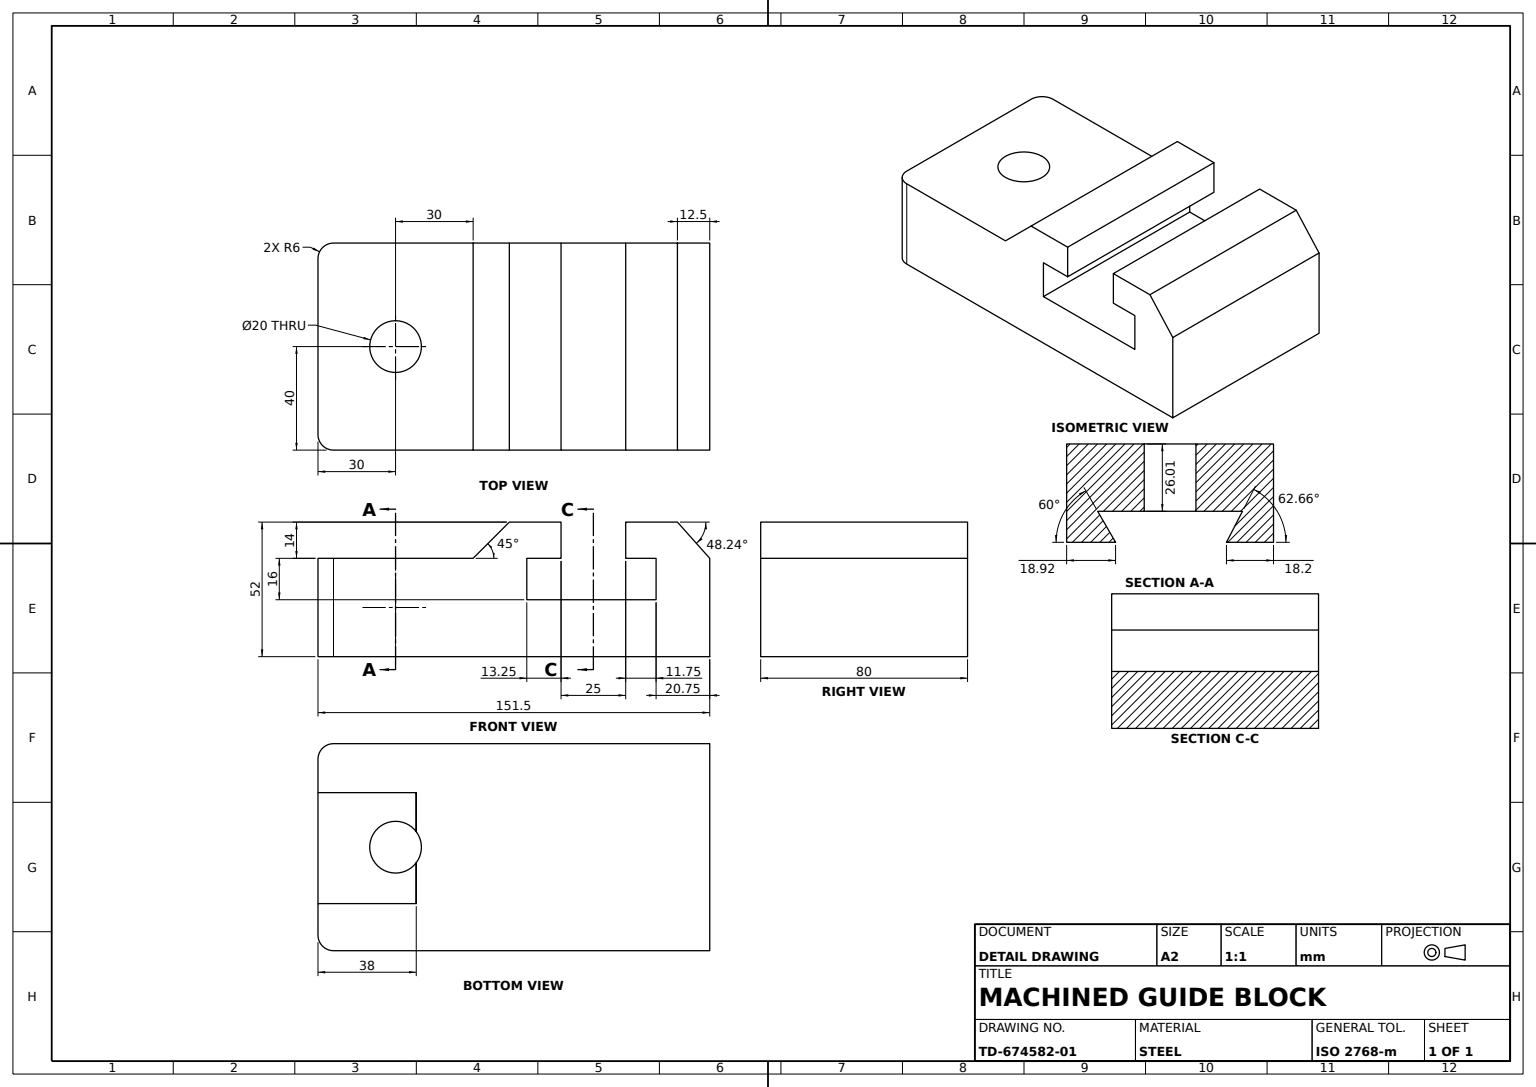
SolidWorks part; units mm, degrees
material "Plain Carbon Steel"
ref_plane "Front Plane" through (0, 0, 0) normal (0, 0, 1) x (1, 0, 0)
ref_plane "Top Plane" through (0, 0, 0) normal (0, 1, 0) x (1, 0, 0)
ref_plane "Right Plane" through (0, 0, 0) normal (1, 0, 0) x (0, 0, -1)
sketch "Base Profile Sketch" plane through (0, 0, 0) normal (0, 0, 1) x (1, 0, 0)
  line L0 (54, 0) -> (144, 0)
  line L1 (131.5, 52) -> (144, 38)
  line L2 (52.5, 0) -> (-1.5, 0)
  line L3 (52.5, 0) -> (54, 0)
  line L4 (144, 38) -> (144, 22)
  line L5 (54, 0) -> (144, 0)
  line L6 (86.5, 52) -> (86.5, 38)
  line L7 (111.5, 52) -> (111.5, 38)
  line L8 (52.5, 0) -> (144, 0)
  line L9 (86.5, 52) -> (66.5, 52)
  line L10 (111.5, 52) -> (131.5, 52)
  line L11 (144, 22) -> (144, 0)
  line L12 (52.5, 38) -> (66.5, 52)
  line L13 (0, 0) -> (0, 0.1905)
  line L14 (52.5, 0) -> (54, 0)
  line L15 (-1.5, 38) -> (-1.5, 0)
  line L16 (86.5, 38) -> (73.25, 38)
  line L17 (73.25, 38) -> (86.5, 38)
  line L18 (123.25, 38) -> (123.25, 22)
  line L19 (123.25, 22) -> (73.25, 22)
  line L20 (73.25, 22) -> (73.25, 38)
  line L21 (111.5, 38) -> (123.25, 38)
  line L22 (52.5, 38) -> (-1.5, 38)
  arc A0 (-1.5, 0) -> (0, 0.1905) centre (-1.5, 6) ccw
  dimension "D1" = 6
  dimension "D2" = 1.5
  dimension "D3" = 54
  dimension "D4" = 55.5
  dimension "D5" = 68
  dimension "D6" = 74.75
  dimension "D7" = 88
  dimension "D8" = 113
  dimension "D9" = 124.75
  dimension "D10" = 145.5
  dimension "D11" = 22
  dimension "D12" = 38
  dimension "D13" = 52
extrude "Base Body" add sketch "Base Profile Sketch" along normal blind 80 contours L15 A0 L13 L2 L3 L0 L11 L4 L1 L10 L7 L21 L18 L19 L20 L16 L6 L9 L12 L22
sketch "Raised Block Sketch" plane through (0, 38, 0) normal (0, 1, 0) x (1, 0, 0)
  line L0 (-1.5, 0) -> (-1.5, -6)
  line L1 (-1.5, -80) -> (-1.5, 0) construction
  line L2 (-1.5, -80) -> (-1.5, -74)
  line L3 (-1.5, -6) -> (-1.5, -74)
  line L4 (-7.5, -6) -> (-7.5, -74)
  arc A0 (-1.5, 0) -> (-7.5, -6) centre (-1.5, -6) ccw
  arc A1 (-7.5, -74) -> (-1.5, -80) centre (-1.5, -74) ccw
  dimension "D1" = 6
extrude "Raised Block" add sketch "Raised Block Sketch" against normal blind 38
sketch "Wedge Sketch" plane through (0, 0, 0) normal (0, 0, -1) x (-1, 0, 0)
  line L0 (0, 0.1905) -> (0, 0)
  line L1 (0, 0) -> (1.5, 0)
  line L2 (1.5, 0) -> (0, 0.1905)
extrude "Wedge Boss" add sketch "Wedge Sketch" against normal blind 80
sketch "Top Hole Sketch" plane through (0, 38, 0) normal (0, 1, 0) x (1, 0, 0)
  line L0 (-7.5, -6) -> (-7.5, -74) construction
  circle A0 centre (22.5, -40) radius 10
  dimension "D1" = 20
  dimension "D2" = 30
  dimension "D3" = 40
extrude "Top Hole" cut sketch "Top Hole Sketch" against normal blind 38
sketch "Profile Cut Sketch" plane through (-7.5, 0, 0) normal (-1, 0, 0) x (0, 0, 1)
  line L0 (6, 38) -> (74, 38) construction
  line L1 (6, 0) -> (74, 0) construction
  line L2 (40, 11.9897) -> (12, 11.9897)
  line L3 (12, 11.9897) -> (68, 11.9897)
  line L4 (68, 11.9897) -> (61.0777, 0)
  line L5 (68, 11.9897) -> (68.0743, 11.9897) construction
  line L6 (61.0777, 0) -> (40, 0)
  line L7 (40, 0) -> (18.2, 0)
  line L8 (18.2, 0) -> (12, 11.9897)
  line M3 (6, 0) -> (74, 0)
  dimension "D1" = 6
  dimension "D2" = 12.2
  dimension "D3" = 55.0777
  dimension "D4" = 26.0103
extrude "Profile Cut" cut sketch "Profile Cut Sketch" against normal blind 38 contours L8 L4 L3 L2 M3
